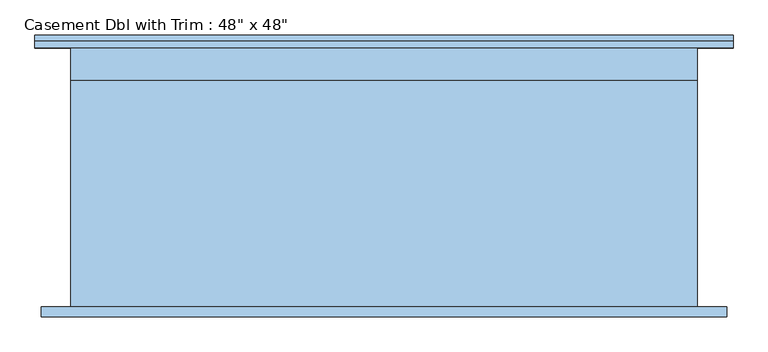
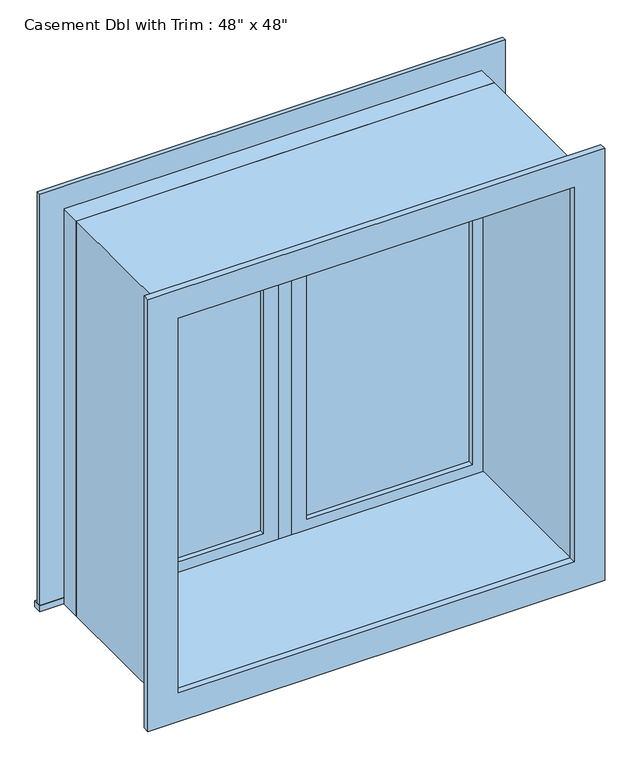
"""IFC4 building model written with IfcOpenShell, lengths in millimetres: window geometry."""

from ifc_helpers import new_model, si_unit, frame, origin, place, context, project, spatial, polyline, outline, extrude, source, transform, mapped, element, save


def window_25ed8443(model_context):
    return source(origin(), model_context, "Body", "SweptSolid", [
        extrude(outline(polyline([(63.5, 236.4225668), (546.1, 236.4225668), (546.1, 223.7225668), (63.5, 223.7225668), (63.5, 236.4225668)])), frame((0.0, 0.0, 977.9), z_axis=(0.0, 0.0, 1.0), x_axis=(1.0, 0.0, 0.0)), (0.0, 0.0, 1.0), 1092.2),
        extrude(outline(polyline([(2114.55, 19.05), (933.45, 19.05), (933.45, 590.55), (2114.55, 590.55), (2114.55, 19.05)]), holes=[polyline([(2070.1, 63.5), (2070.1, 546.1), (977.9, 546.1), (977.9, 63.5), (2070.1, 63.5)])]), frame((0.0, 207.8475668, 0.0), z_axis=(0.0, 1.0, 0.0), x_axis=(0.0, 0.0, 1.0)), (0.0, 0.0, 1.0), 44.45),
        extrude(outline(polyline([(19.05, 207.8475668), (-19.05, 207.8475668), (-19.05, 271.3475668), (19.05, 271.3475668), (19.05, 207.8475668)])), frame((0.0, 0.0, 933.45), z_axis=(0.0, 0.0, 1.0), x_axis=(1.0, 0.0, 0.0)), (0.0, 0.0, 1.0), 1181.1),
        extrude(outline(polyline([(-679.45, 296.7475668), (679.45, 296.7475668), (679.45, 271.3475668), (-679.45, 271.3475668), (-679.45, 296.7475668)])), frame((0.0, 0.0, 914.4), z_axis=(0.0, 0.0, 1.0), x_axis=(1.0, 0.0, 0.0)), (0.0, 0.0, 1.0), 19.05),
        extrude(outline(polyline([(2114.55, -590.55), (2114.55, 590.55), (933.45, 590.55), (933.45, 679.45), (2203.45, 679.45), (2203.45, -679.45), (933.45, -679.45), (933.45, -590.55), (2114.55, -590.55)])), frame((0.0, 271.3475668, 0.0), z_axis=(0.0, 1.0, 0.0), x_axis=(0.0, 0.0, 1.0)), (0.0, 0.0, 1.0), 12.7),
        extrude(outline(polyline([(2190.75, 666.75), (2190.75, -666.75), (857.25, -666.75), (857.25, 666.75), (2190.75, 666.75)]), holes=[polyline([(2101.85, 577.85), (946.15, 577.85), (946.15, -577.85), (2101.85, -577.85), (2101.85, 577.85)])]), frame((0.0, -252.2975668, 0.0), z_axis=(0.0, 1.0, 0.0), x_axis=(0.0, 0.0, 1.0)), (0.0, 0.0, 1.0), 19.05),
        extrude(outline(polyline([(-63.5, 223.7225668), (-546.1, 223.7225668), (-546.1, 236.4225668), (-63.5, 236.4225668), (-63.5, 223.7225668)])), frame((0.0, 0.0, 977.9), z_axis=(0.0, 0.0, 1.0), x_axis=(1.0, 0.0, 0.0)), (0.0, 0.0, 1.0), 1092.2),
        extrude(outline(polyline([(2114.55, -590.55), (933.45, -590.55), (933.45, -19.05), (2114.55, -19.05), (2114.55, -590.55)]), holes=[polyline([(2070.1, -546.1), (2070.1, -63.5), (977.9, -63.5), (977.9, -546.1), (2070.1, -546.1)])]), frame((0.0, 207.8475668, 0.0), z_axis=(0.0, 1.0, 0.0), x_axis=(0.0, 0.0, 1.0)), (0.0, 0.0, 1.0), 44.45),
        extrude(outline(polyline([(2133.6, -609.6), (914.4, -609.6), (914.4, 609.6), (2133.6, 609.6), (2133.6, -609.6)]), holes=[polyline([(2101.85, -577.85), (2101.85, 577.85), (946.15, 577.85), (946.15, -577.85), (2101.85, -577.85)])]), frame((0.0, -233.2475668, 0.0), z_axis=(0.0, 1.0, 0.0), x_axis=(0.0, 0.0, 1.0)), (0.0, 0.0, 1.0), 441.0951336),
        extrude(outline(polyline([(2133.6, 609.6), (2133.6, -609.6), (914.4, -609.6), (914.4, 609.6), (2133.6, 609.6)]), holes=[polyline([(2114.55, 590.55), (933.45, 590.55), (933.45, -590.55), (2114.55, -590.55), (2114.55, 590.55)])]), frame((0.0, 207.8475668, 0.0), z_axis=(0.0, 1.0, 0.0), x_axis=(0.0, 0.0, 1.0)), (0.0, 0.0, 1.0), 63.5),
    ])


if __name__ == "__main__":
    model = new_model("IFC4")
    model_context = context("Model", 3, world=origin())
    ifc_project = project(units=[si_unit("LENGTHUNIT", "METRE", prefix="MILLI")], contexts=[model_context])
    site = spatial("IfcSite", under=ifc_project)
    building = spatial("IfcBuilding", under=site)
    placement = place(None, origin())
    window_shape = window_25ed8443(model_context)
    element("IfcWindow", 1, ObjectType="Casement Dbl with Trim : 48\" x 48\"", at=placement, inside=building, context=model_context, shape_type="MappedRepresentation", body=[
        mapped(window_shape, transform((0.0, 0.0, 0.0), x_axis=(1.0, 0.0, 0.0), y_axis=(0.0, 1.0, 0.0), z_axis=(0.0, 0.0, 1.0))),
    ])
    save(model, "model.ifc")

# Revit data of these elements
# Type "Casement Dbl with Trim : 48\" x 48\""
#   Type Mark = "13"
#   Construction Type Id = "GSP4R"
#   Assembly Code = "B2020100"
#   Analytic Construction = "1/8 in Pilkington single glazing"
#   Visual Light Transmittance = 0.9
#   Solar Heat Gain Coefficient = 0.78
#   Heat Transfer Coefficient (U) = 0.6496 BTU/(h·ft²·°F)
#   Height = 4' - 0"
#   Default Sill Height = 3' - 0"
#   Trim Projection - Ext. = 0' - 0 1/2"
#   Trim Projection - Int. = 0' - 0 3/4"
#   Trim Width - Exterior = 0' - 3 1/2"
#   Trim Width - Interior = 0' - 3 1/2"
#   Width = 4' - 0"
#   Window Inset = 0' - 0 3/4"
#   Define Thermal Properties by = 1
#   Glass Pane Material = Glass
#   Sash Material = Sash
#   Trim Exterior Material = Trim
#   Trim Interior Material = Trim
#   Wall Closure = (empty or 0)
# Element 1 (IfcWindow, "Casement Dbl with Trim : 48\" x 48\"")
#   Materials on its faces: "Sash", "Trim", "Glass"
# Materials
#   "Glass": class "Glass", colour RGB 0 128 192, transparency 0.75, Description = "Soda Lime Glass", Cost = 0
#   "Sash": class "Wood", colour RGB 224 178 126, transparency 0
#   "Trim": class "Wood", colour RGB 224 178 126, transparency 0
